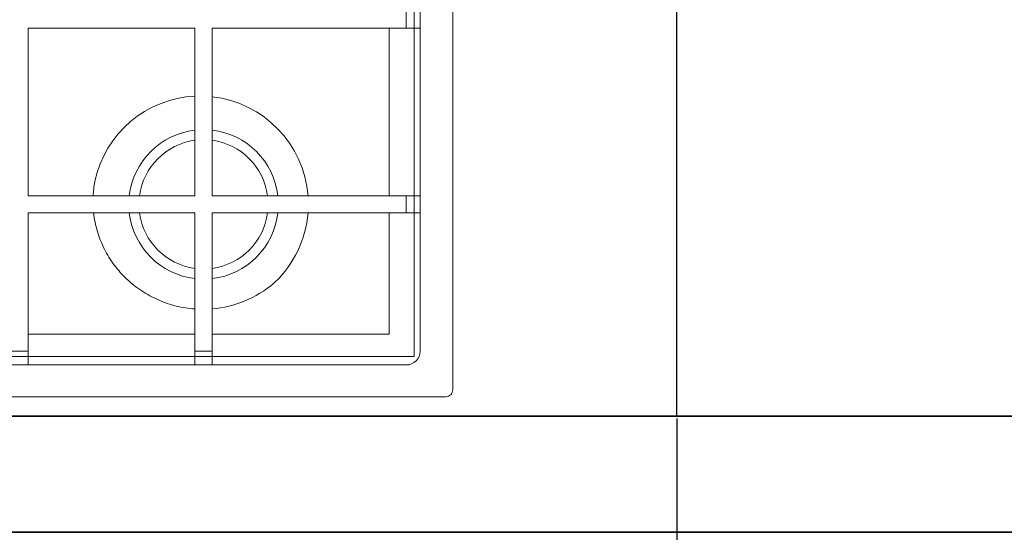
# Model space of a CAD drawing. Units: inches. Extents: x -1198 to -69, y -512 to 437.
# Tile 31 of 50: x -635 to -610, y 158 to 171. Entities that reach past the tile are written whole.
import ezdxf

# ---------------------------------------------------------------- set-up
doc = ezdxf.new("R2010")
doc.units = ezdxf.units.IN
doc.header["$MEASUREMENT"] = 0
for name, color, linetype, lineweight in [('0_Pen_No__7', 7, 'Continuous', 18), ('A-ANNO-DIMS', 2, 'Continuous', 18), ('A-EQPM', 60, 'Continuous', 18), ('A-FLOR-CASE', 7, 'Continuous', 25), ('A-WALL', 7, 'Continuous', 35)]:
    doc.layers.add(name, color=color, linetype=linetype, lineweight=lineweight)
doc.styles.get("Standard").update_dxf_attribs({"font": 'arial.ttf'})
doc.dimstyles.get("Standard").update_dxf_attribs({"dimtxt": 6, "dimasz": 6, "dimexe": 0.18, "dimexo": 0.0625, "dimgap": 0.09, "dimtad": 0, "dimtih": 1, "dimtoh": 1, "dimdec": 0, "dimzin": 0, "dimdsep": 46, "dimlunit": 4, "dimtxsty": 'Standard', "dimblk": 'OBLIQUE', "dimcen": 0.09, "dimadec": 0, "dimazin": 0, "dimtfac": 1, "dimtdec": 0, "dimtofl": 0, "dimtmove": 0, "dimatfit": 3, "dimfxl": 1, "dimtolj": 1, "dimtzin": 0, "dimarcsym": 0})

# ---------------------------------------------------------------- blocks, each defined once
blk = doc.blocks.new('new block')
at = {"layer": '0_Pen_No__7'}
for p, q in [((-201.32, 567.06), (-190.06, 567.06)), ((-80.82, 567.06), (-69.55, 567.06)), ((-190.06, 555.8), (-80.82, 555.8)), ((-328.59, 465.14), (-328.59, 476.4)), ((-317.33, 355.33), (-317.33, 465.14)), ((-328.59, 344.07), (-328.59, 355.33))]:
    blk.add_line(p, q, dxfattribs=at)
for points in [[(-354.49, 596.91), (481.18, 596.91, -0.414214), (485.68, 592.4), (485.68, 99.11), (486.24, 99.11), (486.24, 95.73), (485.68, 95.73), (485.68, 4.5, -0.414214), (481.18, 0), (-354.49, 0, -0.414214), (-359, 4.5), (-359, 95.73), (-359.56, 95.73), (-359.56, 99.11), (-359, 99.11), (-359, 592.4, -0.414214)], [(464.28, 132.33), (464.28, 567.06, 0.414214), (455.27, 576.07), (-328.59, 576.07, 0.414214), (-337.6, 567.06), (-337.6, 132.33, 0.414214), (-328.59, 123.32), (455.27, 123.32, 0.414214)]]:
    blk.add_lwpolyline(points, format="xyb", close=True, dxfattribs=at)
for points in [[(-201.32, 576.07), (-201.32, 476.4), (-337.6, 476.4)], [(-80.82, 576.07), (-80.82, 476.4), (-190.06, 476.4), (-190.06, 576.07)], [(-317.33, 476.4), (-317.33, 555.8), (-201.32, 555.8)], [(-123.65, 476.4), (-123.84, 477.94), (-124.06, 479.47), (-124.32, 481), (-124.61, 482.53), (-124.94, 484.04), (-125.29, 485.55), (-125.69, 487.05), (-126.11, 488.55), (-126.57, 490.03), (-127.06, 491.5), (-127.58, 492.96), (-128.14, 494.41), (-128.73, 495.84), (-129.35, 497.26), (-130, 498.67), (-130.68, 500.06), (-131.4, 501.44), (-132.14, 502.8), (-132.91, 504.15), (-133.71, 505.47), (-134.55, 506.78), (-135.4, 508.08), (-136.29, 509.35), (-137.21, 510.6), (-138.15, 511.83), (-139.12, 513.04), (-140.11, 514.23), (-141.14, 515.4), (-142.18, 516.54), (-143.25, 517.67), (-144.35, 518.76), (-145.46, 519.84), (-146.61, 520.89), (-147.77, 521.92), (-148.95, 522.92), (-150.16, 523.89), (-151.39, 524.84), (-152.63, 525.76), (-153.9, 526.66), (-155.19, 527.52), (-156.49, 528.36), (-157.81, 529.18), (-159.15, 529.96), (-160.51, 530.71), (-161.88, 531.44), (-163.26, 532.14), (-164.66, 532.8), (-166.08, 533.44), (-167.51, 534.05), (-168.95, 534.62), (-170.4, 535.17), (-171.86, 535.68), (-173.34, 536.16), (-174.82, 536.62), (-176.31, 537.04), (-177.82, 537.42), (-179.33, 537.78), (-180.85, 538.1), (-182.37, 538.4), (-183.9, 538.65), (-185.43, 538.88), (-186.97, 539.07), (-188.52, 539.23), (-190.06, 539.36)], [(-337.6, 465.14), (-201.32, 465.14), (-201.32, 355.33), (-337.6, 355.33)]]:
    blk.add_lwpolyline(points, dxfattribs=at)
for points in [[(-333.7, 12.95), (460.3, 12.95), (460.3, 570.44), (-333.7, 570.44)], [(-190.06, 355.33), (-190.06, 465.14), (-80.82, 465.14), (-80.82, 355.33)]]:
    blk.add_lwpolyline(points, close=True, dxfattribs=at)
for centre, radius, start, end in [((-195.46, 468.12), 71.42, 94.71073, 130.2725), ((-193.79, 470.71), 70.6, 133.55313, 175.37917), ((-195.69, 470.77), 48.99, 96.60065, 173.39935), ((-228.93, 507.66), 19.61, 130.34198, 133.52793), ((-195.69, 470.77), 48.99, 6.60065, 83.39935), ((-195.69, 470.77), 42.35, 97.64264, 172.3569), ((-195.69, 470.77), 42.35, 7.6431, 82.35736), ((-193.46, 470.72), 70.94, 184.51789, 263.6357), ((-195.69, 470.77), 48.99, 186.60065, 263.39935), ((-195.69, 470.77), 42.35, 187.6431, 262.35736), ((-195.69, 470.77), 48.99, 276.60065, 353.39935), ((-195.69, 470.77), 42.35, 277.64264, 352.3569), ((-192.72, 468.81), 69.49, 349.39254, 356.96894), ((-193.31, 470.1), 70.32, 272.64753, 348.10391), ((-142.89, 459.48), 18.78, 348.1147, 349.39229)]:
    blk.add_arc(centre, radius, start, end, dxfattribs=at)
blk = doc.blocks.new('COUNTER-L')
at = {"ltscale": 10}
blk.add_line((49.349, 0), (49.349, 24), dxfattribs=at)
blk = doc.blocks.new('_Oblique')
at = {"color": 0, "linetype": 'ByBlock', "lineweight": -2}
blk.add_line((-0.5, -0.5), (0.5, 0.5), dxfattribs=at)
blk = doc.blocks.new('*D56')
at = {"layer": 'A-ANNO-DIMS', "color": 0, "lineweight": -2, "ltscale": 10, "transparency": 16777216}
for p, q in [((-618.339, 257.228), (-603.822, 257.228)), ((-604.002, 257.228), (-604.002, 212.422)), ((-604.002, 161.228), (-604.002, 206.033)), ((-618.339, 161.228), (-603.822, 161.228))]:
    blk.add_line(p, q, dxfattribs=at)
at = {"layer": 'DEFPOINTS', "color": 0, "ltscale": 10, "transparency": 16777216}
for p in [(-618.402, 257.228), (-604.002, 257.228), (-618.402, 161.228)]:
    blk.add_point(p, dxfattribs=at)
at = {"layer": 'A-ANNO-DIMS', "color": 0, "lineweight": -2, "ltscale": 10, "transparency": 16777216, "xscale": 6, "yscale": 6, "zscale": 6}
for p, rotation in [((-604.002, 257.228), 90), ((-604.002, 161.228), 270)]:
    blk.add_blockref('_Oblique', p, dxfattribs=dict(at, rotation=rotation))
at = {"layer": 'A-ANNO-DIMS', "color": 0, "ltscale": 10, "transparency": 16777216, "insert": (-604.002, 209.228), "char_height": 6, "attachment_point": 5}
blk.add_mtext('\\A1;COUNTER 96 TYP.', dxfattribs=at)
blk = doc.blocks.new('*D57')
at = {"layer": 'A-ANNO-DIMS', "color": 0, "lineweight": -2, "ltscale": 10, "transparency": 16777216}
for p, q in [((-667.751, 161.165), (-667.751, 146.648)), ((-618.402, 161.165), (-618.402, 146.648)), ((-667.751, 146.828), (-657.89, 146.828)), ((-618.402, 146.828), (-628.263, 146.828))]:
    blk.add_line(p, q, dxfattribs=at)
at = {"layer": 'DEFPOINTS', "color": 0, "ltscale": 10, "transparency": 16777216}
for p in [(-667.751, 161.228), (-618.402, 161.228), (-618.402, 146.828)]:
    blk.add_point(p, dxfattribs=at)
at = {"layer": 'A-ANNO-DIMS', "color": 0, "lineweight": -2, "ltscale": 10, "transparency": 16777216, "xscale": 6, "yscale": 6, "zscale": 6, "rotation": 180}
blk.add_blockref('_Oblique', (-667.751, 146.828), dxfattribs=at)
at = {"layer": 'A-ANNO-DIMS', "color": 0, "lineweight": -2, "ltscale": 10, "transparency": 16777216, "xscale": 6, "yscale": 6, "zscale": 6}
blk.add_blockref('_Oblique', (-618.402, 146.828), dxfattribs=at)
at = {"layer": 'A-ANNO-DIMS', "color": 0, "ltscale": 10, "transparency": 16777216, "insert": (-643.076, 146.828), "char_height": 6, "attachment_point": 5}
blk.add_mtext('\\A1;49 TYP.', dxfattribs=at)

msp = doc.modelspace()

# ---------------------------------------------------------------- linework, layer by layer
at = {"layer": 'A-WALL', "ltscale": 10}
for p, q in [((-565.7509, 161.2277), (-691.7509, 161.2277)), ((-571.7509, 158.2277), (-691.7509, 158.2277))]:
    msp.add_line(p, q, dxfattribs=at)

# ---------------------------------------------------------------- block references
at = {"layer": 'A-EQPM', "xscale": 0.0393700787401575, "yscale": 0.0393700787401575, "zscale": 0.0393700787401575, "rotation": 180}
msp.add_blockref('new block', (-638.3186, 185.2277), dxfattribs=at)
at = {"layer": 'A-FLOR-CASE'}
msp.add_blockref('COUNTER-L', (-667.751, 161.228), dxfattribs=at)

# ---------------------------------------------------------------- dimensions: what is measured, and where the dimension line sits
at = {"layer": 'A-ANNO-DIMS', "ltscale": 10}
dim = msp.add_linear_dim(base=(-604.0019, 257.2277), p1=(-618.4019, 161.2277), p2=(-618.4019, 257.2277), angle=90, text='COUNTER <> TYP.', dimstyle='Standard', override={"dimdec": 0, "dimlfac": 1, "dimrnd": 0, "dimzin": 0, "dimdsep": 46, "dimlunit": 2}, dxfattribs=at)
dim.commit()
dim.dimension.update_dxf_attribs({"geometry": '*D56', "text_midpoint": (-604.0019, 209.2277)})
dim = msp.add_linear_dim(base=(-618.4019, 146.8277), p1=(-667.7509, 161.2277), p2=(-618.4019, 161.2277), text='<> TYP.', dimstyle='Standard', override={"dimdec": 0, "dimlfac": 1, "dimrnd": 0, "dimzin": 0, "dimdsep": 46, "dimlunit": 2}, dxfattribs=at)
dim.commit()
dim.dimension.update_dxf_attribs({"geometry": '*D57', "text_midpoint": (-643.0764, 146.8277)})

doc.saveas('drawing.dxf')
